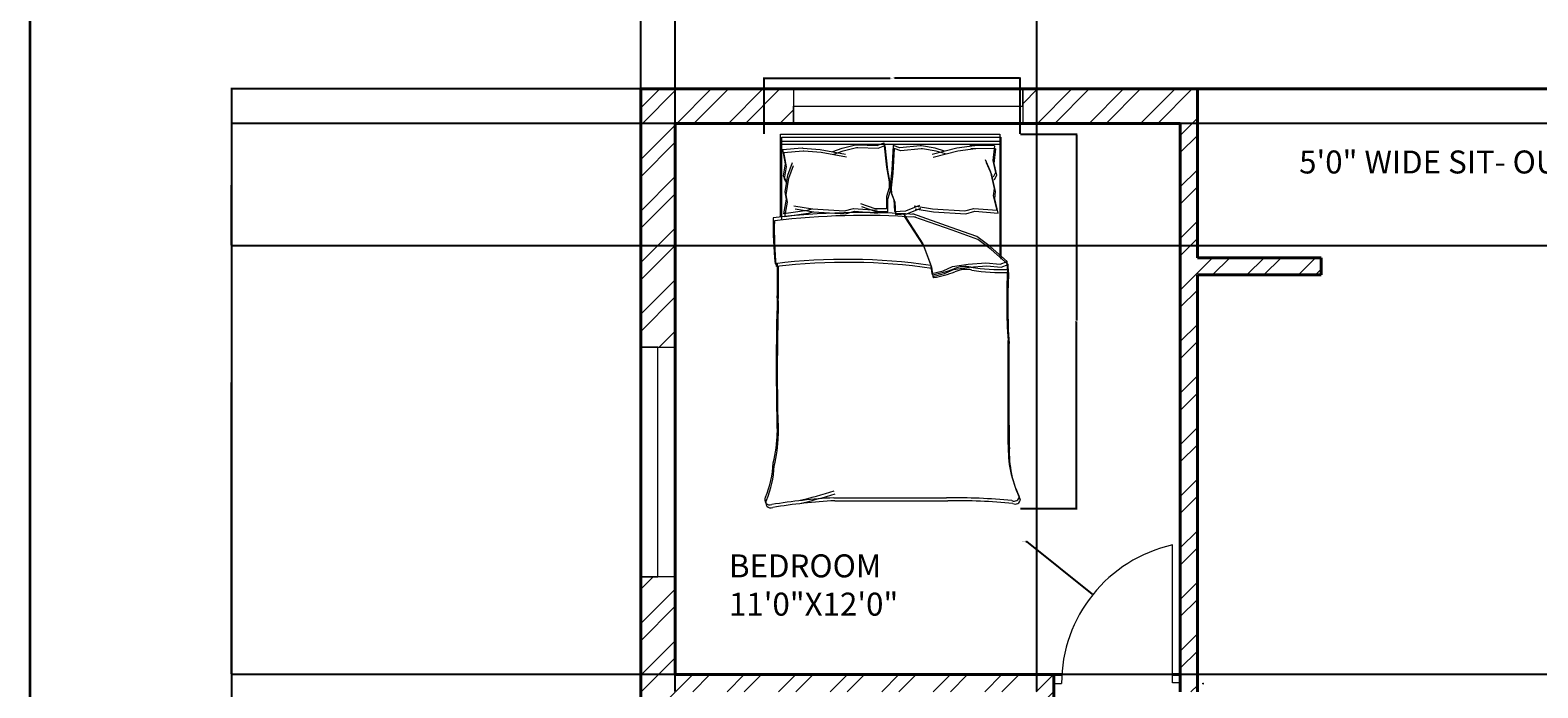
# Model space of a CAD drawing. Units: inches. Extents: x 1355 to 2746, y 1171 to 2751.
# Tile 10 of 24: x 1355 to 1749, y 1983 to 2155. Entities that reach past the tile are written whole.
import ezdxf

# ---------------------------------------------------------------- set-up
doc = ezdxf.new("R2010")
doc.units = ezdxf.units.IN
for name, color, linetype, lineweight in [('A-ANNO-DIMS', 2, 'Continuous', 18), ('A-ANNO-TTLB', 7, 'Continuous', 35), ('A-AREA-IDEN', 7, 'Continuous', 18), ('A-DOOR', 3, 'Continuous', 20), ('A-FURN', 8, 'Continuous', 13), ('A-GLAZ', 4, 'Continuous', 18), ('A-WALL', 7, 'Continuous', 40), ('A-WALL-PATT', 252, 'Continuous', 13)]:
    doc.layers.add(name, color=color, linetype=linetype, lineweight=lineweight)
doc.styles.get("Standard").update_dxf_attribs({"font": 'arial.ttf'})
doc.dimstyles.get("Standard").update_dxf_attribs({"dimtxt": 0.18, "dimasz": 0.18, "dimexe": 0.18, "dimexo": 0.0625, "dimgap": 0.09, "dimtad": 0, "dimtih": 1, "dimtoh": 1, "dimdec": 4, "dimzin": 0, "dimdsep": 46, "dimtxsty": 'Standard', "dimcen": 0.09, "dimadec": 0, "dimazin": 0, "dimtfac": 1, "dimtdec": 4, "dimtofl": 0, "dimtmove": 0, "dimatfit": 3, "dimfxl": 1, "dimtolj": 1, "dimtzin": 0, "dimarcsym": 0})

# ---------------------------------------------------------------- blocks, each defined once
blk = doc.blocks.new('BED-DOUBLE-PLAN')
for p, q in [((75.16, 62.38), (96.87, 62.38)), ((75.93, 62.66), (97.64, 62.66)), ((76.95, 55.42), (76.08, 61.53)), ((76.08, 61.53), (79.9, 60.84)), ((77.72, 55.7), (76.85, 61.81)), ((76.85, 61.81), (80.66, 61.11)), ((78.9, 59.17), (78.1, 54.34)), ((79.9, 60.84), (81.8, 61.19)), ((80.66, 61.11), (82.57, 61.46)), ((81.8, 61.19), (86.14, 60.49)), ((82.57, 61.46), (86.9, 60.77)), ((85.96, 61.71), (84.75, 61.01)), ((86.73, 61.98), (85.52, 61.29)), ((89.08, 61.19), (85.96, 61.71)), ((86.14, 60.49), (89.43, 59.28)), ((89.85, 61.46), (86.73, 61.98)), ((86.9, 60.77), (90.2, 59.55)), ((92.9, 61.88), (89.08, 61.19)), ((93.66, 62.15), (89.85, 61.46)), ((92.87, 61.87), (93.27, 56.74)), ((93.64, 62.15), (94.03, 57.02)), ((95.03, 62.38), (95.03, 5.09)), ((95.8, 62.66), (95.8, 5.36)), ((96.87, 62.38), (96.87, 5.09)), ((97.64, 62.66), (97.64, 5.36)), ((77.34, 54.06), (76.95, 55.42)), ((78.14, 58.9), (77.34, 54.06)), ((78.1, 54.34), (77.72, 55.7)), ((93.24, 56.62), (92.9, 52.03)), ((93.27, 56.74), (93.24, 56.62)), ((94.01, 56.89), (93.66, 52.31)), ((94.03, 57.02), (94.01, 56.89)), ((77.34, 54.06), (76.82, 45.66)), ((78.1, 54.34), (77.59, 45.93)), ((92.9, 52.03), (91.68, 45.45)), ((93.66, 52.31), (92.45, 45.72)), ((1.87, 48.49), (1.87, 18.98)), ((2.64, 48.76), (2.64, 19.26)), ((92.38, 48.74), (93.24, 46.31)), ((93.14, 49.01), (94.01, 46.59)), ((76.82, 45.66), (77.49, 43.31)), ((77.59, 45.93), (78.25, 43.58)), ((78.25, 43.58), (77.77, 37.43)), ((93.24, 46.31), (94.11, 42.85)), ((94.01, 46.59), (94.88, 43.12)), ((77.49, 43.31), (77, 37.16)), ((77.38, 37.65), (78.68, 41.42)), ((78.14, 37.93), (79.45, 41.7)), ((94.11, 42.46), (93.94, 37.13)), ((94.11, 42.85), (94.11, 42.46)), ((94.88, 42.74), (94.7, 37.41)), ((94.88, 43.12), (94.88, 42.74)), ((77.38, 34.71), (77.38, 37.65)), ((78.14, 34.98), (78.14, 37.93)), ((95.4, 35.67), (88.98, 34.98)), ((93.94, 37.13), (94.63, 35.4)), ((94.7, 37.41), (95.4, 35.67)), ((79.83, 32.82), (76.62, 32.62)), ((76.62, 32.62), (76.8, 29.68)), ((80.59, 34.71), (77.38, 34.71)), ((80.6, 33.1), (77.39, 32.9)), ((77.39, 32.9), (77.57, 29.96)), ((81.36, 34.98), (78.14, 34.98)), ((82.03, 33.66), (79.83, 32.82)), ((82.84, 34.01), (80.59, 34.71)), ((82.8, 33.93), (80.6, 33.1)), ((83.61, 34.29), (81.36, 34.98)), ((83.59, 33.75), (82.03, 33.66)), ((84.36, 34.03), (82.8, 33.93)), ((84.4, 34.01), (82.84, 34.01)), ((87.44, 33.3), (83.59, 33.75)), ((85.17, 34.29), (83.61, 34.29)), ((88.21, 33.57), (84.36, 34.03)), ((88.22, 34.71), (84.4, 34.01)), ((88.98, 34.98), (85.17, 34.29)), ((93.89, 33.01), (87.44, 33.3)), ((94.65, 33.28), (88.21, 33.57)), ((94.63, 35.4), (88.22, 34.71)), ((93.3, 31.24), (93.89, 33.01)), ((94.07, 31.51), (94.65, 33.28)), ((76.03, 30.27), (68.25, 25.25)), ((76.8, 30.55), (69.01, 25.52)), ((72.52, 17.82), (76.03, 27.82)), ((73.28, 18.1), (76.8, 28.09)), ((76.8, 29.68), (78.34, 26)), ((77.57, 29.96), (79.11, 26.28)), ((78.9, 27.78), (78.1, 22.95)), ((93.81, 25.93), (93.3, 31.24)), ((94.57, 26.2), (94.07, 31.51)), ((68.25, 25.25), (62.87, 23.21)), ((69.01, 25.52), (63.63, 23.48)), ((78.14, 27.51), (77.34, 22.68)), ((93.18, 22.03), (93.83, 25.54)), ((93.83, 25.54), (93.81, 25.93)), ((93.95, 22.3), (94.6, 25.82)), ((94.6, 25.82), (94.57, 26.2)), ((62.87, 23.21), (60.45, 22.84)), ((60.45, 22.84), (61.2, 19.86)), ((61.2, 19.86), (62.31, 17.45)), ((63.63, 23.48), (61.22, 23.11)), ((61.22, 23.11), (61.96, 20.14)), ((61.96, 20.14), (63.08, 17.72)), ((77.34, 22.68), (76.82, 14.27)), ((78.1, 22.95), (77.59, 14.54)), ((93.19, 16.3), (91.57, 22.8)), ((93.96, 16.57), (92.34, 23.07)), ((92.47, 19.55), (93.18, 22.03)), ((93.23, 19.83), (93.95, 22.3)), ((62.31, 17.45), (62.87, 13.37)), ((63.08, 17.72), (63.63, 13.64)), ((70.1, 11.14), (72.52, 17.82)), ((70.87, 11.41), (73.28, 18.1)), ((93.82, 11.75), (93.19, 16.3)), ((94.59, 12.02), (93.96, 16.57)), ((62.87, 13.37), (63.24, 8.72)), ((63.63, 13.64), (64, 9)), ((76.82, 14.27), (77.49, 11.92)), ((77.49, 11.92), (77, 5.77)), ((77.59, 14.54), (78.25, 12.19)), ((78.25, 12.19), (77.77, 6.04)), ((93.81, 6.47), (93.92, 12.95)), ((93.92, 12.95), (93.82, 11.75)), ((94.57, 6.75), (94.69, 13.22)), ((94.69, 13.22), (94.59, 12.02)), ((63.24, 8.72), (62.87, 5.01)), ((64, 9), (63.63, 5.28)), ((64.38, 3.44), (68.27, 7.88)), ((67.51, 7.61), (70.1, 11.14)), ((68.27, 7.88), (70.87, 11.41)), ((86.97, 7.43), (90.18, 8.85)), ((87.74, 7.71), (90.95, 9.12)), ((62.87, 5.01), (63.61, 3.17)), ((63.61, 3.17), (67.51, 7.61)), ((63.63, 5.28), (64.38, 3.44)), ((96.87, 5.09), (64.97, 5.09)), ((97.64, 5.36), (65.74, 5.36)), ((77, 5.77), (80.77, 6.7)), ((77.77, 6.04), (81.53, 6.97)), ((80.77, 6.7), (82.69, 6.47)), ((81.53, 6.97), (83.46, 6.75)), ((82.69, 6.47), (86.97, 7.43)), ((83.46, 6.75), (87.74, 7.71)), ((86.88, 6.21), (85.62, 6.83)), ((87.64, 6.49), (86.39, 7.1)), ((89.96, 6.93), (86.88, 6.21)), ((90.72, 7.2), (87.64, 6.49)), ((93.81, 6.47), (89.96, 6.93)), ((94.57, 6.75), (90.72, 7.2)), ((61.52, 3.07), (63.61, 3.17, 4.64)), ((62.28, 3.35), (64.38, 3.44, 4.64))]:
    blk.add_line(p, q)
for centre, radius, start, end in [((1.3, 65.24), 1.31, 56.1736, 203.4781), ((-143.9, 40.86), 145.97, 2.9958, 9.4091), ((2.07, 65.52), 1.31, 56.1736, 203.4781), ((-143.14, 41.13), 145.97, 2.9958, 9.4091), ((12.62, 92.52), 28.25, 247.9751, 266.652), ((13.39, 92.79), 28.25, 247.9751, 266.652), ((19.53, 98.8), 35.53, 256.0648, 268.9113), ((20.29, 99.07), 35.53, 256.0648, 268.9113), ((36.19, -514.68), 578.22, 88.22771, 91.71854), ((36.96, -514.41), 578.22, 88.22771, 91.71854), ((59.5, 267.13), 203.94, 268.4762, 271.0082), ((60.27, 267.4), 203.94, 268.4762, 271.0082), ((-90.53, 45.26), 154.68, 351.7845, 6.9006), ((72.78, -35.55), 99.87, 88.7218, 95.604), ((-89.76, 45.54), 154.68, 351.7845, 6.9006), ((73.55, -35.27), 99.87, 88.7218, 95.604), ((-121.38, 40.94), 197.77, 356.0865, 6.7821), ((-120.62, 41.22), 197.77, 356.0865, 6.7821), ((125.3, 87.2), 127.63, 193.3832, 197.7053), ((126.07, 87.47), 127.63, 193.3832, 197.7053), ((60.38, 22.63), 0.221, 70.2464, 181.1377), ((95.1, 29.2), 35.55, 190.6617, 199.8806), ((61.15, 22.9), 0.221, 70.2464, 181.1377), ((95.86, 29.47), 35.55, 190.6617, 199.8806), ((-157.62, 17.21), 159.5, 354.4998, 0.6351), ((-156.85, 17.49), 159.5, 354.4998, 0.6351), ((54.83, 14.11), 7.46, 348.6608, 23.7384), ((55.6, 14.38), 7.46, 348.6608, 23.7384), ((104.85, 5.01), 43.38, 169.8763, 182.5657), ((105.62, 5.29), 43.38, 169.8763, 182.5657), ((2.32, 1.32), 1.32, 152.6588, 266.02), ((3.08, 1.59), 1.32, 152.6588, 266.02), ((14.55, -24.75), 27.65, 87.4714, 116.4681), ((15.32, -24.48), 27.65, 87.4714, 116.4681), ((15.56, 5471.89), 5469.02, 270.00217, 270.28689), ((16.33, 5472.16), 5469.02, 270.00217, 270.28689), ((53.34, -151.96), 155.25, 86.9791, 93.8365), ((54.1, -151.69), 155.25, 86.9791, 93.8365)]:
    blk.add_arc(centre, radius, start, end)
blk = doc.blocks.new('WINDOW-PLAN-60')
for p, q in [((0, 60), (9, 60)), ((9, 60), (4.5, 60)), ((4.5, 60), (4.5, 0)), ((4.5, 0), (0, 0)), ((0, 0), (9, 0))]:
    blk.add_line(p, q)
blk = doc.blocks.new('WINDOW-PLAN-60-2')
for p, q in [((4.5, 60), (0, 60)), ((0, 60), (9, 60)), ((4.5, 0), (4.5, 60)), ((9, 0), (0, 0)), ((0, 0), (4.5, 0))]:
    blk.add_line(p, q)
blk = doc.blocks.new('DOOR-BED-NW')
for p, q in [((31, 0.16), (31, 36.16)), ((33, 0.16), (31, 0.16)), ((0, 0), (2, 0))]:
    blk.add_line(p, q)
blk.add_arc((39.05, 0), 37.05, 102.5441, 180)
blk = doc.blocks.new('*D33')
at = {"layer": 'A-ANNO-DIMS', "color": 0, "lineweight": -2, "transparency": 16777216}
for p, q in [((1614, 2127.5), (1628.78, 2127.5)), ((1628.6, 2127.32), (1628.6, 2078.8)), ((1628.6, 2029.91), (1628.6, 2078.43)), ((1614, 2029.73), (1628.78, 2029.73))]:
    blk.add_line(p, q, dxfattribs=at)
at = {"layer": 'A-ANNO-DIMS', "color": 0, "transparency": 16777216}
for points in [[(1628.57, 2127.32), (1628.63, 2127.32), (1628.6, 2127.5)], [(1628.57, 2029.91), (1628.63, 2029.91), (1628.6, 2029.73)]]:
    blk.add_solid(points, dxfattribs=at)
at = {"layer": 'Defpoints', "color": 0, "transparency": 16777216}
for p in [(1613.93, 2127.5), (1628.6, 2127.5), (1613.93, 2029.73)]:
    blk.add_point(p, dxfattribs=at)
at = {"layer": 'A-ANNO-DIMS', "color": 0, "transparency": 16777216, "insert": (1628.6, 2078.62), "char_height": 0.18, "attachment_point": 5}
blk.add_mtext('\\A1;BED 98 TYP.', dxfattribs=at)
blk = doc.blocks.new('*D34')
at = {"layer": 'A-ANNO-DIMS', "color": 0, "lineweight": -2, "transparency": 16777216}
for p, q in [((1547.01, 2127.56), (1547.01, 2142.34)), ((1547.19, 2142.16), (1579.94, 2142.16)), ((1613.75, 2142.16), (1581, 2142.16)), ((1613.93, 2127.56), (1613.93, 2142.34))]:
    blk.add_line(p, q, dxfattribs=at)
at = {"layer": 'A-ANNO-DIMS', "color": 0, "transparency": 16777216}
for points in [[(1547.19, 2142.19), (1547.19, 2142.13), (1547.01, 2142.16)], [(1613.75, 2142.19), (1613.75, 2142.13), (1613.93, 2142.16)]]:
    blk.add_solid(points, dxfattribs=at)
at = {"layer": 'Defpoints', "color": 0, "transparency": 16777216}
for p in [(1547.01, 2142.16), (1547.01, 2127.5), (1613.93, 2127.5)]:
    blk.add_point(p, dxfattribs=at)
at = {"layer": 'A-ANNO-DIMS', "color": 0, "transparency": 16777216, "insert": (1580.47, 2142.16), "char_height": 0.18, "attachment_point": 5}
blk.add_mtext('\\A1;67 TYP.', dxfattribs=at)
blk = doc.blocks.new('*D95')
at = {"layer": 'A-ANNO-DIMS', "color": 0, "lineweight": -2, "transparency": 16777216}
for p, q in [((1514.71, 2139.36), (1514.71, 2716.58)), ((1514.89, 2716.4), (1727.42, 2716.4)), ((1940.53, 2716.4), (1728, 2716.4)), ((1940.71, 2139.36), (1940.71, 2716.58))]:
    blk.add_line(p, q, dxfattribs=at)
at = {"layer": 'A-ANNO-DIMS', "color": 0, "transparency": 16777216}
for points in [[(1514.89, 2716.43), (1514.89, 2716.37), (1514.71, 2716.4)], [(1940.53, 2716.43), (1940.53, 2716.37), (1940.71, 2716.4)]]:
    blk.add_solid(points, dxfattribs=at)
at = {"layer": 'Defpoints', "color": 0, "transparency": 16777216}
for p in [(1940.71, 2716.4), (1514.71, 2139.3), (1940.71, 2139.3)]:
    blk.add_point(p, dxfattribs=at)
at = {"layer": 'A-ANNO-DIMS', "color": 0, "transparency": 16777216, "insert": (1727.71, 2716.4), "char_height": 0.18, "attachment_point": 5}
blk.add_mtext('\\A1;426', dxfattribs=at)
blk = doc.blocks.new('*D96')
at = {"layer": 'A-ANNO-DIMS', "color": 0, "lineweight": -2, "transparency": 16777216}
for p, q in [((1514.65, 2139.3), (1407.53, 2139.3)), ((1407.71, 2139.12), (1407.71, 1725.48)), ((1407.71, 1311.48), (1407.71, 1725.12)), ((1514.65, 1311.3), (1407.53, 1311.3))]:
    blk.add_line(p, q, dxfattribs=at)
at = {"layer": 'A-ANNO-DIMS', "color": 0, "transparency": 16777216}
for points in [[(1407.68, 2139.12), (1407.74, 2139.12), (1407.71, 2139.3)], [(1407.68, 1311.48), (1407.74, 1311.48), (1407.71, 1311.3)]]:
    blk.add_solid(points, dxfattribs=at)
at = {"layer": 'Defpoints', "color": 0, "transparency": 16777216}
for p in [(1407.71, 2139.3), (1514.71, 2139.3), (1514.71, 1311.3)]:
    blk.add_point(p, dxfattribs=at)
at = {"layer": 'A-ANNO-DIMS', "color": 0, "transparency": 16777216, "insert": (1407.71, 1725.3), "char_height": 0.18, "attachment_point": 5}
blk.add_mtext('\\A1;828', dxfattribs=at)
blk = doc.blocks.new('*D104')
at = {"layer": 'A-ANNO-DIMS', "color": 0, "lineweight": -2, "transparency": 16777216}
for p, q in [((2089.33, 1986.3), (1407.53, 1986.3)), ((1407.71, 1986.12), (1407.71, 1951.98)), ((1407.71, 1917.48), (1407.71, 1951.62)), ((2089.33, 1917.3), (1407.53, 1917.3))]:
    blk.add_line(p, q, dxfattribs=at)
at = {"layer": 'A-ANNO-DIMS', "color": 0, "transparency": 16777216}
for points in [[(1407.68, 1986.12), (1407.74, 1986.12), (1407.71, 1986.3)], [(1407.68, 1917.48), (1407.74, 1917.48), (1407.71, 1917.3)]]:
    blk.add_solid(points, dxfattribs=at)
at = {"layer": 'Defpoints', "color": 0, "transparency": 16777216}
for p in [(1407.71, 1986.3), (2089.39, 1986.3), (2089.39, 1917.3)]:
    blk.add_point(p, dxfattribs=at)
at = {"layer": 'A-ANNO-DIMS', "color": 0, "transparency": 16777216, "insert": (1407.71, 1951.8), "char_height": 0.18, "attachment_point": 5}
blk.add_mtext('\\A1;69', dxfattribs=at)
blk = doc.blocks.new('*D105')
at = {"layer": 'A-ANNO-DIMS', "color": 0, "lineweight": -2, "transparency": 16777216}
for p, q in [((2080.33, 2139.3), (1407.53, 2139.3)), ((1407.71, 2139.12), (1407.71, 2062.98)), ((1407.71, 1986.48), (1407.71, 2062.62)), ((2089.33, 1986.3), (1407.53, 1986.3))]:
    blk.add_line(p, q, dxfattribs=at)
at = {"layer": 'A-ANNO-DIMS', "color": 0, "transparency": 16777216}
for points in [[(1407.68, 2139.12), (1407.74, 2139.12), (1407.71, 2139.3)], [(1407.68, 1986.48), (1407.74, 1986.48), (1407.71, 1986.3)]]:
    blk.add_solid(points, dxfattribs=at)
at = {"layer": 'Defpoints', "color": 0, "transparency": 16777216}
for p in [(1407.71, 2139.3), (2080.39, 2139.3), (2089.39, 1986.3)]:
    blk.add_point(p, dxfattribs=at)
at = {"layer": 'A-ANNO-DIMS', "color": 0, "transparency": 16777216, "insert": (1407.71, 2062.8), "char_height": 0.18, "attachment_point": 5}
blk.add_mtext('\\A1;153', dxfattribs=at)
blk = doc.blocks.new('*D111')
at = {"layer": 'A-ANNO-DIMS', "color": 0, "lineweight": -2, "transparency": 16777216}
for p, q in [((2497.33, 2130.3), (1407.53, 2130.3)), ((1407.71, 2130.12), (1407.71, 2114.5)), ((1407.71, 2098.51), (1407.71, 2114.14)), ((2497.33, 2098.33), (1407.53, 2098.33))]:
    blk.add_line(p, q, dxfattribs=at)
at = {"layer": 'A-ANNO-DIMS', "color": 0, "transparency": 16777216}
for points in [[(1407.68, 2130.12), (1407.74, 2130.12), (1407.71, 2130.3)], [(1407.68, 2098.51), (1407.74, 2098.51), (1407.71, 2098.33)]]:
    blk.add_solid(points, dxfattribs=at)
at = {"layer": 'Defpoints', "color": 0, "transparency": 16777216}
for p in [(1407.71, 2130.3), (2497.39, 2130.3), (2497.39, 2098.33)]:
    blk.add_point(p, dxfattribs=at)
at = {"layer": 'A-ANNO-DIMS', "color": 0, "transparency": 16777216, "insert": (1407.71, 2114.32), "char_height": 0.18, "attachment_point": 5}
blk.add_mtext('\\A1;31.97', dxfattribs=at)
blk = doc.blocks.new('*D135')
at = {"layer": 'A-ANNO-DIMS', "color": 0, "lineweight": -2, "transparency": 16777216}
for p, q in [((1523.71, 1981.86), (1523.71, 2716.58)), ((1523.89, 2716.4), (1570.63, 2716.4)), ((1618.03, 2716.4), (1571.28, 2716.4)), ((1618.21, 1981.86), (1618.21, 2716.58))]:
    blk.add_line(p, q, dxfattribs=at)
at = {"layer": 'A-ANNO-DIMS', "color": 0, "transparency": 16777216}
for points in [[(1523.89, 2716.43), (1523.89, 2716.37), (1523.71, 2716.4)], [(1618.03, 2716.43), (1618.03, 2716.37), (1618.21, 2716.4)]]:
    blk.add_solid(points, dxfattribs=at)
at = {"layer": 'Defpoints', "color": 0, "transparency": 16777216}
for p in [(1618.21, 2716.4), (1523.71, 1981.8), (1618.21, 1981.8)]:
    blk.add_point(p, dxfattribs=at)
at = {"layer": 'A-ANNO-DIMS', "color": 0, "transparency": 16777216, "insert": (1570.96, 2716.4), "char_height": 0.18, "attachment_point": 5}
blk.add_mtext('\\A1;94.5', dxfattribs=at)
blk = doc.blocks.new('*D152')
at = {"layer": 'A-ANNO-DIMS', "color": 0, "lineweight": -2, "transparency": 16777216}
for p, q in [((1615.33, 2021.09), (1615.51, 2021.09)), ((1615.51, 2021.09), (1632.71, 2007.29)), ((1661.66, 1984), (1661.84, 1984)), ((1661.75, 1983.91), (1661.75, 1984.09))]:
    blk.add_line(p, q, dxfattribs=at)
at = {"layer": 'A-ANNO-DIMS', "color": 0, "transparency": 16777216}
blk.add_solid([(1632.73, 2007.32), (1632.69, 2007.27), (1632.85, 2007.18)], dxfattribs=at)
at = {"layer": 'Defpoints', "color": 0, "transparency": 16777216}
for p in [(1632.85, 2007.18), (1661.75, 1984)]:
    blk.add_point(p, dxfattribs=at)
at = {"layer": 'A-ANNO-DIMS', "color": 0, "transparency": 16777216, "insert": (1614.78, 2021.09), "char_height": 0.18, "attachment_point": 5}
blk.add_mtext('\\A1;R37.046', dxfattribs=at)

msp = doc.modelspace()

# ---------------------------------------------------------------- hatches: boundary and pattern name
at = {"layer": 'A-WALL-PATT'}
h = msp.add_hatch(dxfattribs=at)
h.set_pattern_fill('ANSI32', color=256)
h.paths.add_polyline_path([(1660.2083, 2139.3018), (1614.5977, 2139.3018), (1614.5977, 2130.3018), (1655.7083, 2130.3018), (1655.7083, 1981.8018), (1660.2083, 1981.8018), (1660.2083, 2090.7225), (1692.5832, 2090.7225), (1692.5832, 2095.2225), (1660.2083, 2095.2225)])
h.paths.add_polyline_path([(1523.7083, 2130.3018), (1554.5977, 2130.3018), (1554.5977, 2134.8018), (1554.5977, 2139.3018), (1514.7083, 2139.3018), (1514.7083, 2071.8385), (1523.7083, 2071.8385)])
h.paths.add_polyline_path([(1940.7083, 2139.3018), (1883.7928, 2139.3018), (1883.7928, 2130.3018), (1931.7083, 2130.3018), (1931.7083, 2098.3333), (1940.7083, 2098.3333)])
h.paths.add_polyline_path([(1799.7083, 2130.3018), (1823.7928, 2130.3018), (1823.7928, 2134.8018), (1823.7928, 2139.3018), (1795.2083, 2139.3018), (1795.2083, 2130.3018), (1795.2083, 2095.2225), (1759.2134, 2095.2225), (1759.2134, 2090.7225), (1795.2083, 2090.7225), (1795.2083, 1981.8018), (1799.7083, 1981.8018), (1799.7083, 1986.3018)])
h.paths.add_polyline_path([(1940.7083, 2038.3333), (1931.7083, 2038.3333), (1931.7083, 1986.3018), (1832.7083, 1986.3018), (1832.7083, 1947.1338), (1837.2083, 1947.1338), (1837.2083, 1981.8018), (1931.7083, 1981.8018), (1931.7083, 1967.1939), (1940.7083, 1967.1939)])
h.paths.add_polyline_path([(1940.7083, 1943.1939), (1931.7083, 1943.1939), (1931.7083, 1921.8018), (1837.2083, 1921.8018), (1837.2083, 1926.0511), (1832.7083, 1926.0511), (1832.7083, 1917.3018), (1931.7083, 1917.3018), (1931.7083, 1908.3321), (1940.7083, 1908.3321)])
h.paths.add_polyline_path([(1940.7083, 1884.3321), (1931.7083, 1884.3321), (1931.7083, 1869.3018), (1899.4583, 1869.3018), (1899.4583, 1864.8018), (1931.7083, 1864.8018), (1931.7083, 1773.3018), (1786.5143, 1773.3018), (1786.5143, 1764.3018), (1844.7083, 1764.3018), (1844.7083, 1748.9343), (1853.7083, 1748.9343), (1853.7083, 1764.3018), (1931.7083, 1764.3018), (1931.7083, 1652.9424), (1940.7083, 1652.9424)])
h.paths.add_polyline_path([(1799.7083, 1864.8018), (1806.0522, 1864.8018), (1806.0522, 1867.0518), (1806.0522, 1869.3018), (1799.7083, 1869.3018), (1799.7083, 1917.3018), (1799.7083, 1921.8018), (1795.2083, 1921.8018), (1795.2083, 1773.3018), (1799.7083, 1773.3018)])
h.paths.add_polyline_path([(1872.8988, 1867.0518), (1872.8988, 1869.3018), (1867.2083, 1869.3018), (1867.2083, 1917.3018), (1862.7083, 1917.3018), (1862.7083, 1869.3018), (1836.9546, 1869.3018), (1836.9546, 1864.8018), (1862.7083, 1864.8018), (1872.8988, 1864.8018)])
h.paths.add_polyline_path([(1749.2197, 1773.3018), (1655.7083, 1773.3018), (1523.7083, 1773.3018), (1523.7083, 1828.4963), (1514.7083, 1828.4963), (1514.7083, 1753.9033), (1519.2083, 1753.9033), (1523.7083, 1753.9033), (1523.7083, 1764.3018), (1655.7083, 1764.3018), (1749.2197, 1764.3018), (1749.2197, 1768.8018)])
h.paths.add_polyline_path([(1660.2083, 1921.8018), (1655.7083, 1921.8018), (1655.7083, 1917.3018), (1655.7083, 1773.3018), (1660.2083, 1773.3018)])
h.paths.add_polyline_path([(1523.7083, 2011.8385), (1514.7083, 2011.8385), (1514.7083, 1973.114), (1519.2083, 1973.114), (1523.7083, 1973.114), (1523.7083, 1976.8227), (1523.7083, 1981.8018), (1618.2083, 1981.8018), (1618.2083, 1921.8018), (1553.707, 1921.8018), (1553.707, 1917.3018), (1622.7083, 1917.3018), (1622.7083, 1919.5518), (1622.7083, 1921.8018), (1622.7083, 1986.3018), (1523.7083, 1986.3018)])
h.paths.add_polyline_path([(1529.6686, 1919.5518), (1529.6686, 1921.8018), (1523.7083, 1921.8018), (1523.7083, 1949.114), (1514.7083, 1949.114), (1514.7083, 1888.4963), (1523.7083, 1888.4963), (1523.7083, 1917.3018), (1529.6686, 1917.3018)])
h.paths.add_polyline_path([(1538.9419, 1775.643), (1585.5504, 1775.643), (1585.5504, 1798.0318), (1538.9419, 1798.0318)], flags=25)
h.paths.add_polyline_path([(1696.7097, 1497.3356), (1769.5651, 1497.3356), (1769.5651, 1523.4559), (1696.7097, 1523.4559)], flags=9)
h.paths.add_polyline_path([(1629.1643, 1230.5133), (1877.0879, 1230.5133), (1877.0879, 1267.606), (1629.1643, 1267.606)], flags=9)
h.paths.add_polyline_path([(2533.4462, 2215.4033), (2579.9292, 2215.4033), (2579.9292, 2231.889), (2533.4462, 2231.889)], flags=9)
h.paths.add_polyline_path([(2540.822, 2515.6945), (2594.2245, 2515.6945), (2594.2245, 2545.5463), (2540.822, 2545.5463)], flags=9)
h.paths.add_polyline_path([(2535.9857, 2588.2819), (2582.4687, 2588.2819), (2582.4687, 2604.7675), (2535.9857, 2604.7675)], flags=9)
h.paths.add_polyline_path([(2537.1627, 2617.1172), (2649.1245, 2617.1172), (2649.1245, 2633.6029), (2537.1627, 2633.6029)], flags=9)
h.paths.add_polyline_path([(2218.0051, 2168.228), (2363.9573, 2168.228), (2363.9573, 2205.3208), (2218.0051, 2205.3208)], flags=9)
h.paths.add_polyline_path([(1650.2156, 2165.3631), (1800.3547, 2165.3631), (1800.3547, 2202.4559), (1650.2156, 2202.4559)], flags=9)
h.paths.add_polyline_path([(2553.9592, 1610.7663), (2588.4203, 1610.7663), (2588.4203, 1660.2233), (2553.9592, 1660.2233)], flags=9)
h.paths.add_polyline_path([(1549.0868, 1648.2033), (1595.6952, 1648.2033), (1595.6952, 1670.5921), (1549.0868, 1670.5921)], flags=9)
h.paths.add_polyline_path([(1546.9525, 1502.0931), (1583.3413, 1502.0931), (1583.3413, 1524.4819), (1546.9525, 1524.4819)], flags=9)
h.paths.add_polyline_path([(1540.7704, 1433.4431), (1587.3788, 1433.4431), (1587.3788, 1455.8319), (1540.7704, 1455.8319)], flags=9)
h.paths.add_polyline_path([(1683.6524, 1321.5269), (1760.6169, 1321.5269), (1760.6169, 1333.8911), (1683.6524, 1333.8911)], flags=9)
h.paths.add_polyline_path([(1832.0485, 1356.0874), (1873.0989, 1356.0874), (1873.0989, 1378.4762), (1832.0485, 1378.4762)], flags=9)
h.paths.add_polyline_path([(1877.9694, 1431.2138), (1926.3827, 1431.2138), (1926.3827, 1453.578), (1877.9694, 1453.578)], flags=9)
h.paths.add_polyline_path([(1847.3106, 1499.8371), (1883.6994, 1499.8371), (1883.6994, 1522.2259), (1847.3106, 1522.2259)], flags=9)
h.paths.add_polyline_path([(1813.7015, 1640.7287), (1860.3099, 1640.7287), (1860.3099, 1663.1175), (1813.7015, 1663.1175)], flags=9)
h.paths.add_polyline_path([(1876.2576, 1710.2471), (1912.9452, 1710.2471), (1912.9452, 1732.6359), (1876.2576, 1732.6359)], flags=25)
h.paths.add_polyline_path([(1695.9163, 1715.3064), (1736.9668, 1715.3064), (1736.9668, 1737.6952), (1695.9163, 1737.6952)], flags=9)
h.paths.add_polyline_path([(1881.8583, 1888.9094), (1930.2717, 1888.9094), (1930.2717, 1911.2737), (1881.8583, 1911.2737)], flags=9)
h.paths.add_polyline_path([(1823.9298, 1798.6431), (1864.9803, 1798.6431), (1864.9803, 1821.0319), (1823.9298, 1821.0319)], flags=25)
h.paths.add_polyline_path([(1845.6062, 1948.1408), (1881.995, 1948.1408), (1881.995, 1970.5296), (1845.6062, 1970.5296)], flags=25)
h.paths.add_polyline_path([(1849.027, 1991.5151), (1895.6355, 1991.5151), (1895.6355, 2013.9039), (1849.027, 2013.9039)], flags=25)
h.paths.add_polyline_path([(1684.9725, 2113.8416), (1764.2658, 2113.8416), (1764.2658, 2126.2058), (1684.9725, 2126.2058)], flags=9)
h.paths.add_polyline_path([(1688.6193, 1913.0676), (1776.2005, 1913.0676), (1776.2005, 1935.4564), (1688.6193, 1935.4564)], flags=9)
h.paths.add_polyline_path([(1571.4689, 1930.9816), (1607.8577, 1930.9816), (1607.8577, 1953.3704), (1571.4689, 1953.3704)], flags=25)
h.paths.add_polyline_path([(1535.3581, 1998.3125), (1581.9665, 1998.3125), (1581.9665, 2020.7014), (1535.3581, 2020.7014)], flags=9)
h = msp.add_hatch(dxfattribs=at)
h.set_pattern_fill('ANSI32', color=256)
h.paths.add_polyline_path([(1749.2197, 1686.3018), (1732.6892, 1686.3018), (1523.7083, 1686.3018), (1523.7083, 1705.9033), (1514.7083, 1705.9033), (1514.7083, 1647.8732), (1519.2083, 1647.8732), (1523.7083, 1647.8732), (1523.7083, 1677.3018), (1655.7083, 1677.3018), (1655.7083, 1528.8018), (1660.2083, 1528.8018), (1660.2083, 1677.3018), (1732.6892, 1677.3018), (1749.2197, 1677.3018)])
h.paths.add_polyline_path([(1931.7083, 1686.3018), (1853.7083, 1686.3018), (1853.7083, 1703.5696), (1844.7083, 1703.5696), (1844.7083, 1686.3018), (1788.0274, 1686.3018), (1788.0274, 1677.3018), (1795.2083, 1677.3018), (1795.2083, 1528.8018), (1799.7083, 1528.8018), (1799.7083, 1677.3018), (1844.7083, 1677.3018), (1931.7083, 1677.3018)])
h.paths.add_polyline_path([(1931.7083, 1533.3018), (1844.7083, 1533.3018), (1832.7083, 1533.3018), (1832.7083, 1531.0518), (1832.7083, 1528.8018), (1832.7083, 1495.7519), (1837.2083, 1495.7519), (1837.2083, 1528.8018), (1931.7083, 1528.8018)])
h.paths.add_polyline_path([(1940.7083, 1592.9424), (1931.7083, 1592.9424), (1931.7083, 1506.7845), (1940.7083, 1506.7845)])
h.paths.add_polyline_path([(1940.7083, 1482.7845), (1936.2083, 1482.7845), (1931.7083, 1482.7845), (1931.7083, 1320.3018), (1880.7083, 1320.3018), (1880.7083, 1311.3018), (1940.7083, 1311.3018)])
h.paths.add_polyline_path([(1931.7083, 1468.8018), (1844.7083, 1468.8018), (1837.2083, 1468.8018), (1837.2083, 1474.34), (1832.7083, 1474.34), (1832.7083, 1468.8018), (1832.7083, 1464.3018), (1844.7083, 1464.3018), (1931.7083, 1464.3018)])
h.paths.add_polyline_path([(1863.8571, 1464.3018), (1859.3571, 1464.3018), (1859.3571, 1404.1662), (1838.1542, 1404.1662), (1838.1542, 1399.8018), (1869.4185, 1399.8018), (1869.4185, 1402.0518), (1869.4185, 1404.3018), (1863.8571, 1404.3018)])
h.paths.add_polyline_path([(1799.7083, 1399.6662), (1805.4082, 1399.6662), (1805.4082, 1401.9162), (1805.4082, 1404.1662), (1799.7083, 1404.1662), (1799.7083, 1464.3018), (1799.7083, 1468.8018), (1795.2083, 1468.8018), (1795.2083, 1356.2098), (1761.2597, 1356.2098), (1761.2597, 1351.7098), (1795.2083, 1351.7098), (1795.2083, 1320.3018), (1795.2083, 1311.3018), (1844.7083, 1311.3018), (1844.7083, 1315.8018), (1844.7083, 1320.3018), (1799.7083, 1320.3018)])
h.paths.add_polyline_path([(1692.9218, 1356.2098), (1660.2083, 1356.2098), (1660.2083, 1430.786), (1657.9583, 1430.786), (1655.7083, 1430.786), (1655.7083, 1320.3018), (1611.934, 1320.3018), (1611.934, 1311.3018), (1660.2083, 1311.3018), (1660.2083, 1351.7098), (1692.9218, 1351.7098)])
h.paths.add_polyline_path([(1523.7083, 1372.653), (1514.7083, 1372.653), (1514.7083, 1311.3018), (1551.934, 1311.3018), (1551.934, 1315.8018), (1551.934, 1320.3018), (1523.7083, 1320.3018)])
h.paths.add_polyline_path([(1523.7083, 1490.9023), (1514.7083, 1490.9023), (1514.7083, 1432.653), (1519.2083, 1432.653), (1523.7083, 1432.653)])
h.paths.add_polyline_path([(1660.2083, 1468.8018), (1622.7083, 1468.8018), (1622.7083, 1473.1566), (1618.2083, 1473.1566), (1618.2083, 1468.8018), (1523.7083, 1468.8018), (1523.7083, 1464.3018), (1655.7083, 1464.3018), (1655.7083, 1460.5634), (1660.2083, 1460.5634)])
h.paths.add_polyline_path([(1523.7083, 1587.8732), (1514.7083, 1587.8732), (1514.7083, 1514.9023), (1519.2083, 1514.9023), (1523.7083, 1514.9023)])
h.paths.add_polyline_path([(1622.7083, 1533.3018), (1523.7083, 1533.3018), (1523.7083, 1528.8018), (1618.2083, 1528.8018), (1618.2083, 1494.4205), (1622.7083, 1494.4205), (1622.7083, 1528.8018)])
h.paths.add_polyline_path([(1696.7097, 1497.3356), (1769.5651, 1497.3356), (1769.5651, 1523.4559), (1696.7097, 1523.4559)], flags=9)
h.paths.add_polyline_path([(1629.1643, 1230.5133), (1877.0879, 1230.5133), (1877.0879, 1267.606), (1629.1643, 1267.606)], flags=9)
h.paths.add_polyline_path([(2533.4462, 2215.4033), (2579.9292, 2215.4033), (2579.9292, 2231.889), (2533.4462, 2231.889)], flags=9)
h.paths.add_polyline_path([(2540.822, 2515.6945), (2594.2245, 2515.6945), (2594.2245, 2545.5463), (2540.822, 2545.5463)], flags=9)
h.paths.add_polyline_path([(2535.9857, 2588.2819), (2582.4687, 2588.2819), (2582.4687, 2604.7675), (2535.9857, 2604.7675)], flags=9)
h.paths.add_polyline_path([(2537.1627, 2617.1172), (2649.1245, 2617.1172), (2649.1245, 2633.6029), (2537.1627, 2633.6029)], flags=9)
h.paths.add_polyline_path([(2218.0051, 2168.228), (2363.9573, 2168.228), (2363.9573, 2205.3208), (2218.0051, 2205.3208)], flags=9)
h.paths.add_polyline_path([(1650.2156, 2165.3631), (1800.3547, 2165.3631), (1800.3547, 2202.4559), (1650.2156, 2202.4559)], flags=9)
h.paths.add_polyline_path([(2553.9592, 1610.7663), (2588.4203, 1610.7663), (2588.4203, 1660.2233), (2553.9592, 1660.2233)], flags=9)
h.paths.add_polyline_path([(1549.0868, 1648.2033), (1595.6952, 1648.2033), (1595.6952, 1670.5921), (1549.0868, 1670.5921)], flags=25)
h.paths.add_polyline_path([(1546.9525, 1502.0931), (1583.3413, 1502.0931), (1583.3413, 1524.4819), (1546.9525, 1524.4819)], flags=25)
h.paths.add_polyline_path([(1540.7704, 1433.4431), (1587.3788, 1433.4431), (1587.3788, 1455.8319), (1540.7704, 1455.8319)], flags=9)
h.paths.add_polyline_path([(1683.6524, 1321.5269), (1760.6169, 1321.5269), (1760.6169, 1333.8911), (1683.6524, 1333.8911)], flags=9)
h.paths.add_polyline_path([(1832.0485, 1356.0874), (1873.0989, 1356.0874), (1873.0989, 1378.4762), (1832.0485, 1378.4762)], flags=9)
h.paths.add_polyline_path([(1877.9694, 1431.2138), (1926.3827, 1431.2138), (1926.3827, 1453.578), (1877.9694, 1453.578)], flags=9)
h.paths.add_polyline_path([(1847.3106, 1499.8371), (1883.6994, 1499.8371), (1883.6994, 1522.2259), (1847.3106, 1522.2259)], flags=25)
h.paths.add_polyline_path([(1813.7015, 1640.7287), (1860.3099, 1640.7287), (1860.3099, 1663.1175), (1813.7015, 1663.1175)], flags=25)
h.paths.add_polyline_path([(1876.2576, 1710.2471), (1912.9452, 1710.2471), (1912.9452, 1732.6359), (1876.2576, 1732.6359)], flags=9)
h.paths.add_polyline_path([(1695.9163, 1715.3064), (1736.9668, 1715.3064), (1736.9668, 1737.6952), (1695.9163, 1737.6952)], flags=9)
h.paths.add_polyline_path([(1881.8583, 1888.9094), (1930.2717, 1888.9094), (1930.2717, 1911.2737), (1881.8583, 1911.2737)], flags=9)
h.paths.add_polyline_path([(1823.9298, 1798.6431), (1864.9803, 1798.6431), (1864.9803, 1821.0319), (1823.9298, 1821.0319)], flags=9)
h.paths.add_polyline_path([(1845.6062, 1948.1408), (1881.995, 1948.1408), (1881.995, 1970.5296), (1845.6062, 1970.5296)], flags=9)
h.paths.add_polyline_path([(1849.027, 1991.5151), (1895.6355, 1991.5151), (1895.6355, 2013.9039), (1849.027, 2013.9039)], flags=9)
h.paths.add_polyline_path([(1684.9725, 2113.8416), (1764.2658, 2113.8416), (1764.2658, 2126.2058), (1684.9725, 2126.2058)], flags=9)
h.paths.add_polyline_path([(1688.6193, 1913.0676), (1776.2005, 1913.0676), (1776.2005, 1935.4564), (1688.6193, 1935.4564)], flags=9)
h.paths.add_polyline_path([(1538.9419, 1775.643), (1585.5504, 1775.643), (1585.5504, 1798.0318), (1538.9419, 1798.0318)], flags=9)
h.paths.add_polyline_path([(1571.4689, 1930.9816), (1607.8577, 1930.9816), (1607.8577, 1953.3704), (1571.4689, 1953.3704)], flags=9)
h.paths.add_polyline_path([(1535.3581, 1998.3125), (1581.9665, 1998.3125), (1581.9665, 2020.7014), (1535.3581, 2020.7014)], flags=9)

# ---------------------------------------------------------------- linework, layer by layer
at = {"layer": 'A-ANNO-TTLB'}
msp.add_lwpolyline([(1355.0901, 2751.4741), (2746.1804, 2751.4741), (2746.1804, 1182.883), (1355.0901, 1182.883)], close=True, dxfattribs=at)
at = {"layer": 'A-WALL'}
for p, q in [((1514.7083, 2139.3018), (1660.2083, 2139.3018)), ((1514.7083, 2139.3018), (1514.7083, 1311.3018)), ((1660.2083, 2095.2225), (1660.2083, 2139.3018)), ((1660.2083, 2139.3018), (1795.2083, 2139.3018)), ((1523.7083, 2130.3018), (1655.7083, 2130.3018)), ((1523.7083, 2130.3018), (1523.7083, 1986.3018)), ((1655.7083, 2130.3018), (1655.7083, 1981.8018)), ((1660.2083, 2130.3018), (1660.2083, 2095.2225)), ((1660.2083, 2095.2225), (1692.5832, 2095.2225)), ((1692.5832, 2095.2225), (1692.5832, 2090.7225)), ((1692.5832, 2090.7225), (1660.2083, 2090.7225)), ((1660.2083, 2090.7225), (1660.2083, 1981.8018)), ((1523.7083, 1986.3018), (1624.7796, 1986.3018)), ((1622.7083, 1986.3018), (1622.7083, 1921.8018)), ((1653.7083, 1986.3018), (1655.7083, 1986.3018))]:
    msp.add_line(p, q, dxfattribs=at)

# ---------------------------------------------------------------- block references
at = {"layer": 'A-DOOR'}
msp.add_blockref('DOOR-BED-NW', (1622.708, 1984.004), dxfattribs=at)
at = {"layer": 'A-FURN', "rotation": 90.00000000000003}
msp.add_blockref('BED-DOUBLE-PLAN', (1613.9343, 2029.8605), dxfattribs=at)
at = {"layer": 'A-GLAZ', "extrusion": (0, 0, -1), "zscale": -1, "rotation": 270}
msp.add_blockref('WINDOW-PLAN-60', (-1614.598, 2139.302), dxfattribs=at)
at = {"layer": 'A-GLAZ'}
msp.add_blockref('WINDOW-PLAN-60-2', (1514.708, 2011.838), dxfattribs=at)

# ---------------------------------------------------------------- texts
at = {"layer": 'A-AREA-IDEN', "char_height": 6, "attachment_point": 1}
for s, width, insert in [('5\'0" WIDE SIT- OUT', 100.672075, (1686.8204, 2123.2243)), ('BEDROOM\\P11\'0"X12\'0"', 152.706174, (1537.7708, 2017.7198))]:
    msp.add_mtext_dynamic_manual_height_columns(s, width=width, gutter_width=12.5, heights=[0], dxfattribs=dict(at, insert=insert))

# ---------------------------------------------------------------- dimensions: what is measured, and where the dimension line sits
at = {"layer": 'A-ANNO-DIMS'}
for base, p1, p2, override, picture, middle in [((1940.7083, 2716.3999), (1514.7083, 2139.3018), (1940.7083, 2139.3018), {"dimdec": 0, "dimlfac": 1, "dimrnd": 0, "dimzin": 0, "dimdsep": 46, "dimlunit": 2}, '*D95', (1727.7083, 2716.3999)), ((1618.2083, 2716.3999), (1523.7083, 1981.8018), (1618.2083, 1981.8018), {"dimdec": 1, "dimlfac": 1, "dimrnd": 0, "dimzin": 0, "dimdsep": 46, "dimlunit": 2}, '*D135', (1570.9583, 2716.3999))]:
    dim = msp.add_linear_dim(base=base, p1=p1, p2=p2, dimstyle='Standard', override=override, dxfattribs=at)
    dim.commit()
    dim.dimension.update_dxf_attribs({"geometry": picture, "text_midpoint": middle})
for base, p1, p2, angle, text, picture, middle in [((1547.0085, 2142.1642), (1613.9339, 2127.4994), (1547.0085, 2127.4994), 180, '<> TYP.', '*D34', (1580.4712, 2142.1642)), ((1628.5986, 2127.4994), (1613.9339, 2029.7342), (1613.9339, 2127.4994), 90, 'BED <> TYP.', '*D33', (1628.5986, 2078.6168))]:
    dim = msp.add_linear_dim(base=base, p1=p1, p2=p2, angle=angle, text=text, dimstyle='Standard', override={"dimdec": 0, "dimlfac": 1, "dimrnd": 0, "dimzin": 0, "dimdsep": 46, "dimlunit": 2}, dxfattribs=at)
    dim.commit()
    dim.dimension.update_dxf_attribs({"geometry": picture, "text_midpoint": middle})
for base, p1, p2, override, picture, middle in [((1407.7083, 2139.3018), (1514.7083, 1311.3018), (1514.7083, 2139.3018), {"dimdec": 0, "dimlfac": 1, "dimrnd": 0, "dimzin": 0, "dimdsep": 46, "dimlunit": 2}, '*D96', (1407.7083, 1725.3018)), ((1407.7083, 2139.3018), (2089.3909, 1986.3018), (2080.3909, 2139.3018), {"dimdec": 0, "dimlfac": 1, "dimrnd": 0, "dimzin": 0, "dimdsep": 46, "dimlunit": 2}, '*D105', (1407.7083, 2062.8018)), ((1407.7083, 2130.3018), (2497.3909, 2098.3333), (2497.3909, 2130.3018), {"dimdec": 2, "dimlfac": 1, "dimrnd": 0, "dimzin": 0, "dimdsep": 46, "dimlunit": 2}, '*D111', (1407.7083, 2114.3176)), ((1407.7083, 1986.3018), (2089.3909, 1917.3018), (2089.3909, 1986.3018), {"dimdec": 0, "dimlfac": 1, "dimrnd": 0, "dimzin": 0, "dimdsep": 46, "dimlunit": 2}, '*D104', (1407.7083, 1951.8018))]:
    dim = msp.add_linear_dim(base=base, p1=p1, p2=p2, angle=90, dimstyle='Standard', override=override, dxfattribs=at)
    dim.commit()
    dim.dimension.update_dxf_attribs({"geometry": picture, "text_midpoint": middle})
dim = msp.add_radius_dim(center=(1661.7544, 1984.0037), mpoint=(1632.8541, 2007.1809), dimstyle='Standard', override={"dimdec": 3, "dimlfac": 1, "dimrnd": 0, "dimzin": 0, "dimdsep": 46, "dimlunit": 2}, dxfattribs=at)
dim.commit()
dim.dimension.update_dxf_attribs({"geometry": '*D152', "text_midpoint": (1614.7842, 2021.0873), "dimtype": 164})

doc.saveas('drawing.dxf')
